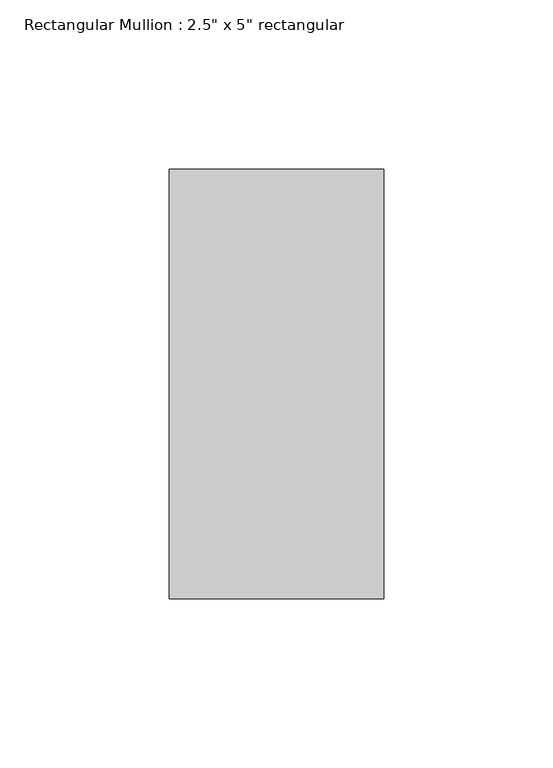
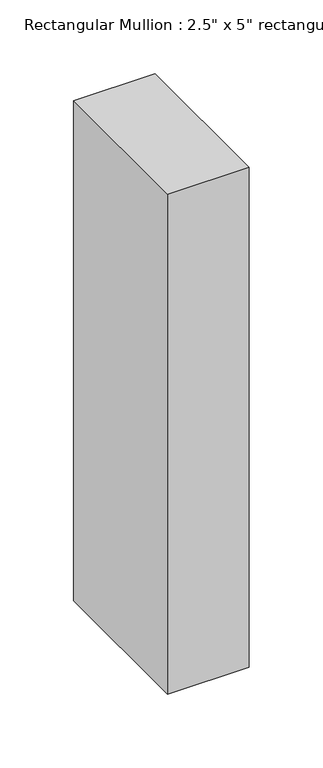
"""IFC4 building model written with IfcOpenShell, lengths in millimetres: member geometry."""

from ifc_helpers import new_model, si_unit, frame, origin, place, context, project, spatial, polyline, outline, extrude, source, transform, mapped, element, save


def member_dc106669(model_context):
    return source(origin(), model_context, "Body", "SweptSolid", [
        extrude(outline(polyline([(0.0, 63.5), (0.0, -63.5), (-63.5, -63.5), (-63.5, 63.5), (0.0, 63.5)])), frame((0.0, 0.0, -412.75), z_axis=(0.0, 0.0, 1.0), x_axis=(1.0, 0.0, 0.0)), (0.0, 0.0, 1.0), 412.75),
    ])


if __name__ == "__main__":
    model = new_model("IFC4")
    model_context = context("Model", 3, world=origin())
    ifc_project = project(units=[si_unit("LENGTHUNIT", "METRE", prefix="MILLI")], contexts=[model_context])
    site = spatial("IfcSite", under=ifc_project)
    building = spatial("IfcBuilding", under=site)
    placement = place(None, origin())
    member_shape = member_dc106669(model_context)
    element("IfcMember", 1, ObjectType="Rectangular Mullion : 2.5\" x 5\" rectangular", at=placement, inside=building, context=model_context, shape_type="MappedRepresentation", body=[
        mapped(member_shape, transform((0.0, 0.0, 0.0), x_axis=(1.0, 0.0, 0.0), y_axis=(0.0, 1.0, 0.0), z_axis=(0.0, 0.0, 1.0))),
    ])
    save(model, "model.ifc")

# Revit data of these elements
# Type "Rectangular Mullion : 2.5\" x 5\" rectangular"
#   built-in parameter 1007304 = 0.416667 (stored number, unit not read)
#   built-in parameter 1007301 = 0.104167 (stored number, unit not read)
#   built-in parameter 1007300 = 0.104167 (stored number, unit not read)
# Element 1 (IfcMember, "Rectangular Mullion : 2.5\" x 5\" rectangular")
#   Materials on its faces: "Rectangle 1 sq"
# Materials
#   "Rectangle 1 sq": class "Generic", colour RGB 120 120 120, transparency 0, Cost = 0
